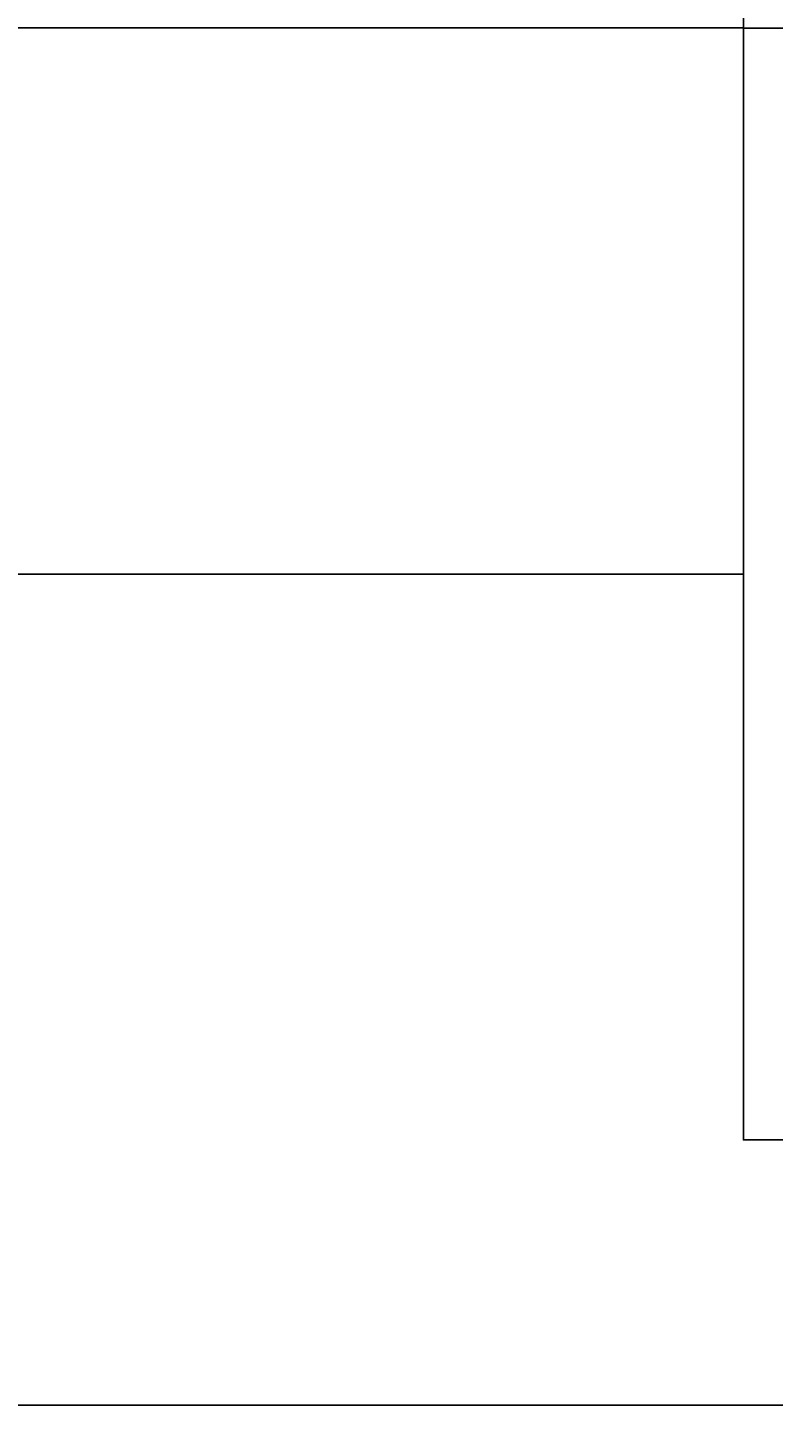
# Model space of a CAD drawing. Units: inches. Extents: x 35362 to 73946, y 43607 to 67532.
# Tile 134 of 134: x 67834 to 68341, y 59170 to 60122. Entities that reach past the tile are written whole.
import ezdxf

# ---------------------------------------------------------------- set-up
doc = ezdxf.new("R2010")
doc.units = ezdxf.units.IN
doc.header["$MEASUREMENT"] = 0
for name, color, linetype, lineweight in [('A-ANNO-DIMS', 2, 'Continuous', 18), ('E-SYMB', 1, 'Continuous', 25), ('E-WIRE', 3, 'Continuous', 25)]:
    doc.layers.add(name, color=color, linetype=linetype, lineweight=lineweight)
doc.styles.get("Standard").update_dxf_attribs({"font": 'arial.ttf'})
doc.dimstyles.get("Standard").update_dxf_attribs({"dimtxt": 0.18, "dimasz": 0.18, "dimexe": 0.18, "dimexo": 0.0625, "dimgap": 0.09, "dimtad": 0, "dimtih": 1, "dimtoh": 1, "dimdec": 4, "dimzin": 0, "dimdsep": 46, "dimtxsty": 'Standard', "dimcen": 0.09, "dimadec": 0, "dimazin": 0, "dimtfac": 1, "dimtdec": 4, "dimtofl": 0, "dimtmove": 0, "dimatfit": 3, "dimfxl": 1, "dimtolj": 1, "dimtzin": 0, "dimarcsym": 0})

# ---------------------------------------------------------------- blocks, each defined once
blk = doc.blocks.new('*D8')
at = {"layer": 'A-ANNO-DIMS', "color": 0, "lineweight": -2, "transparency": 16777216}
for p, q in [((66271.28651900003, 65771.51172800003), (73945.82566600003, 65771.51172800003)), ((73945.64566600005, 65771.33172800003), (73945.64566600005, 59737.03093663782)), ((73945.64566600005, 53702.36633900002), (73945.64566600005, 59736.66713036224)), ((72185.70816600003, 53702.18633900003), (73945.82566600003, 53702.18633900003))]:
    blk.add_line(p, q, dxfattribs=at)
at = {"layer": 'A-ANNO-DIMS', "color": 0, "transparency": 16777216}
for points in [[(73945.61566600006, 65771.33172800003), (73945.67566600005, 65771.33172800003), (73945.64566600005, 65771.51172800003)], [(73945.61566600006, 53702.36633900002), (73945.67566600005, 53702.36633900002), (73945.64566600005, 53702.18633900003)]]:
    blk.add_solid(points, dxfattribs=at)
at = {"layer": 'Defpoints', "color": 0, "transparency": 16777216}
for p in [(66271.22401900003, 65771.51172800003), (73945.64566600005, 65771.51172800003), (72185.64566600003, 53702.18633900003)]:
    blk.add_point(p, dxfattribs=at)
at = {"layer": 'A-ANNO-DIMS', "color": 0, "transparency": 16777216, "insert": (73945.64566600005, 59736.84903349999), "char_height": 0.18, "attachment_point": 5}
blk.add_mtext('\\A1;12069', dxfattribs=at)
blk = doc.blocks.new('*D10')
at = {"layer": 'A-ANNO-DIMS', "color": 0, "lineweight": -2, "transparency": 16777216}
for p, q in [((61240.96983600002, 59185.14395700003), (73945.82566600003, 59185.14395700003)), ((73945.64566600005, 59184.96395700003), (73945.64566600005, 56268.51827402935)), ((73945.64566600005, 53351.70866200003), (73945.64566600005, 56268.1543449707)), ((61240.96983600002, 53351.52866200003), (73945.82566600003, 53351.52866200003))]:
    blk.add_line(p, q, dxfattribs=at)
at = {"layer": 'A-ANNO-DIMS', "color": 0, "transparency": 16777216}
for points in [[(73945.61566600006, 59184.96395700003), (73945.67566600005, 59184.96395700003), (73945.64566600005, 59185.14395700003)], [(73945.61566600006, 53351.70866200003), (73945.67566600005, 53351.70866200003), (73945.64566600005, 53351.52866200003)]]:
    blk.add_solid(points, dxfattribs=at)
at = {"layer": 'Defpoints', "color": 0, "transparency": 16777216}
for p in [(61240.90733600002, 59185.14395700003), (61240.90733600002, 53351.52866200003), (73945.64566600005, 53351.52866200003)]:
    blk.add_point(p, dxfattribs=at)
at = {"layer": 'A-ANNO-DIMS', "color": 0, "transparency": 16777216, "insert": (73945.64566600005, 56268.33630949999), "char_height": 0.18, "attachment_point": 5}
blk.add_mtext('\\A1;5834', dxfattribs=at)
blk = doc.blocks.new('*D35')
at = {"layer": 'A-ANNO-DIMS', "color": 0, "lineweight": -2, "transparency": 16777216}
for p, q in [((61240.907336, 59185.206457), (61240.907336, 67531.691728)), ((61241.08733599999, 67531.51172799998), (64780.42646373397, 67531.51172799998)), ((68320.69076200001, 67531.51172799998), (64781.35163426603, 67531.51172799998)), ((68320.870762, 60122.408832), (68320.870762, 67531.691728))]:
    blk.add_line(p, q, dxfattribs=at)
at = {"layer": 'A-ANNO-DIMS', "color": 0, "transparency": 16777216}
for points in [[(61241.08733599999, 67531.541728), (61241.08733599999, 67531.481728), (61240.907336, 67531.51172799998)], [(68320.69076200001, 67531.541728), (68320.69076200001, 67531.481728), (68320.870762, 67531.51172799998)]]:
    blk.add_solid(points, dxfattribs=at)
at = {"layer": 'Defpoints', "color": 0, "transparency": 16777216}
for p in [(68320.870762, 67531.51172799998), (68320.870762, 60122.346332), (61240.907336, 59185.14395699999)]:
    blk.add_point(p, dxfattribs=at)
at = {"layer": 'A-ANNO-DIMS', "color": 0, "transparency": 16777216, "insert": (64780.889049, 67531.51172799998), "char_height": 0.18, "attachment_point": 5}
blk.add_mtext('\\A1;7080.0', dxfattribs=at)
blk = doc.blocks.new('*D36')
at = {"layer": 'A-ANNO-DIMS', "color": 0, "lineweight": -2, "transparency": 16777216}
for p, q in [((68320.80826200004, 60122.34633200002), (35361.76908500003, 60122.34633200002)), ((35361.94908500003, 60122.16633200002), (35361.94908500003, 57247.82893113781)), ((35361.94908500003, 54373.12772400002), (35361.94908500003, 57247.46512486223)), ((68320.80826200004, 54372.94772400003), (35361.76908500003, 54372.94772400002))]:
    blk.add_line(p, q, dxfattribs=at)
at = {"layer": 'A-ANNO-DIMS', "color": 0, "transparency": 16777216}
for points in [[(35361.91908500003, 60122.16633200002), (35361.97908500003, 60122.16633200002), (35361.94908500003, 60122.34633200002)], [(35361.91908500003, 54373.12772400002), (35361.97908500003, 54373.12772400002), (35361.94908500003, 54372.94772400002)]]:
    blk.add_solid(points, dxfattribs=at)
at = {"layer": 'Defpoints', "color": 0, "transparency": 16777216}
for p in [(68320.87076200004, 60122.34633200002), (35361.94908500003, 54372.94772400002), (68320.87076200004, 54372.94772400003)]:
    blk.add_point(p, dxfattribs=at)
at = {"layer": 'A-ANNO-DIMS', "color": 0, "transparency": 16777216, "insert": (35361.94908500004, 57247.64702799999), "char_height": 0.18, "attachment_point": 5}
blk.add_mtext('\\A1;5749.4', dxfattribs=at)
blk = doc.blocks.new('*D69')
at = {"layer": 'A-ANNO-DIMS', "color": 0, "lineweight": -2, "transparency": 16777216}
for p, q in [((68320.870762, 60122.408832), (68320.870762, 67531.691728)), ((68321.050762, 67531.51172799998), (69913.30289879469, 67531.51172799998)), ((71506.482539, 67531.51172799998), (69914.23040220531, 67531.51172799998)), ((71506.662539, 59451.647447), (71506.662539, 67531.691728))]:
    blk.add_line(p, q, dxfattribs=at)
at = {"layer": 'A-ANNO-DIMS', "color": 0, "transparency": 16777216}
for points in [[(68321.050762, 67531.541728), (68321.050762, 67531.481728), (68320.870762, 67531.51172799998)], [(71506.482539, 67531.541728), (71506.482539, 67531.481728), (71506.662539, 67531.51172799998)]]:
    blk.add_solid(points, dxfattribs=at)
at = {"layer": 'Defpoints', "color": 0, "transparency": 16777216}
for p in [(71506.662539, 67531.51172799998), (68320.870762, 60122.346332), (71506.662539, 59451.584947)]:
    blk.add_point(p, dxfattribs=at)
at = {"layer": 'A-ANNO-DIMS', "color": 0, "transparency": 16777216, "insert": (69913.76665050001, 67531.51172799998), "char_height": 0.18, "attachment_point": 5}
blk.add_mtext('\\A1;3185.8', dxfattribs=at)
blk = doc.blocks.new('*D70')
at = {"layer": 'A-ANNO-DIMS', "color": 0, "lineweight": -2, "transparency": 16777216}
for p, q in [((60785.27513900002, 64923.75242000003), (73945.82566600003, 64923.75242000003)), ((73945.64566600005, 64923.57242000003), (73945.64566600005, 62054.63015302935)), ((73945.64566600005, 59185.32395700003), (73945.64566600005, 62054.26622397069)), ((61240.96983600002, 59185.14395700003), (73945.82566600003, 59185.14395700003))]:
    blk.add_line(p, q, dxfattribs=at)
at = {"layer": 'A-ANNO-DIMS', "color": 0, "transparency": 16777216}
for points in [[(73945.61566600006, 64923.57242000003), (73945.67566600005, 64923.57242000003), (73945.64566600005, 64923.75242000003)], [(73945.61566600006, 59185.32395700003), (73945.67566600005, 59185.32395700003), (73945.64566600005, 59185.14395700003)]]:
    blk.add_solid(points, dxfattribs=at)
at = {"layer": 'Defpoints', "color": 0, "transparency": 16777216}
for p in [(60785.21263900002, 64923.75242000003), (73945.64566600005, 64923.75242000003), (61240.90733600002, 59185.14395700003)]:
    blk.add_point(p, dxfattribs=at)
at = {"layer": 'A-ANNO-DIMS', "color": 0, "transparency": 16777216, "insert": (73945.64566600005, 62054.44818849999), "char_height": 0.18, "attachment_point": 5}
blk.add_mtext('\\A1;5738.6', dxfattribs=at)
blk = doc.blocks.new('*D71')
at = {"layer": 'A-ANNO-DIMS', "color": 0, "lineweight": -2, "transparency": 16777216}
for p, q in [((63159.24181700003, 64828.55626700002), (73945.82566600003, 64828.55626700002)), ((73945.64566600005, 64828.37626700002), (73945.64566600005, 62007.03207652936)), ((73945.64566600005, 59185.32395700003), (73945.64566600005, 62006.6681474707)), ((61240.96983600002, 59185.14395700003), (73945.82566600003, 59185.14395700003))]:
    blk.add_line(p, q, dxfattribs=at)
at = {"layer": 'A-ANNO-DIMS', "color": 0, "transparency": 16777216}
for points in [[(73945.61566600006, 64828.37626700002), (73945.67566600005, 64828.37626700002), (73945.64566600005, 64828.55626700002)], [(73945.61566600006, 59185.32395700003), (73945.67566600005, 59185.32395700003), (73945.64566600005, 59185.14395700003)]]:
    blk.add_solid(points, dxfattribs=at)
at = {"layer": 'Defpoints', "color": 0, "transparency": 16777216}
for p in [(63159.17931700003, 64828.55626700002), (73945.64566600005, 64828.55626700002), (61240.90733600002, 59185.14395700003)]:
    blk.add_point(p, dxfattribs=at)
at = {"layer": 'A-ANNO-DIMS', "color": 0, "transparency": 16777216, "insert": (73945.64566600005, 62006.85011199999), "char_height": 0.18, "attachment_point": 5}
blk.add_mtext('\\A1;5643.4', dxfattribs=at)

msp = doc.modelspace()

# ---------------------------------------------------------------- linework, layer by layer
at = {"layer": 'E-SYMB'}
msp.add_lwpolyline([(68320.87076221016, 60122.34633153839), (68737.80188109005, 60122.34633153839), (68737.80188109005, 59365.72803786365), (68320.87076221016, 59365.72803786365)], close=True, dxfattribs=at)
at = {"layer": 'E-WIRE'}
msp.add_line((68320.87076221016, 59750.68874003685), (64849.6346681835, 59750.68874003685), dxfattribs=at)

# ---------------------------------------------------------------- dimensions: what is measured, and where the dimension line sits
at = {"layer": 'A-ANNO-DIMS'}
for base, p1, p2, picture, middle in [((68320.870762, 67531.51172799998), (61240.907336, 59185.14395699999), (68320.870762, 60122.346332), '*D35', (64780.889049, 67531.51172799998)), ((71506.662539, 67531.51172799998), (68320.870762, 60122.346332), (71506.662539, 59451.584947), '*D69', (69913.76665050001, 67531.51172799998))]:
    dim = msp.add_linear_dim(base=base, p1=p1, p2=p2, dimstyle='Standard', override={"dimdec": 1, "dimlfac": 1, "dimrnd": 0, "dimzin": 0, "dimdsep": 46, "dimlunit": 2}, dxfattribs=at)
    dim.commit()
    dim.dimension.update_dxf_attribs({"geometry": picture, "text_midpoint": middle})
for base, p1, p2, override, picture, middle in [((73945.64566600005, 65771.51172800003), (72185.645666, 53702.186339), (66271.224019, 65771.51172799998), {"dimdec": 0, "dimlfac": 1, "dimrnd": 0, "dimzin": 0, "dimdsep": 46, "dimlunit": 2}, '*D8', (73945.64566600005, 59736.84903349999)), ((73945.64566600005, 64923.75242000003), (61240.907336, 59185.14395699999), (60785.21263899999, 64923.75241999999), {"dimdec": 1, "dimlfac": 1, "dimrnd": 0, "dimzin": 0, "dimdsep": 46, "dimlunit": 2}, '*D70', (73945.64566600005, 62054.44818849999)), ((73945.64566600005, 64828.55626700002), (61240.907336, 59185.14395699999), (63159.179317, 64828.556267), {"dimdec": 1, "dimlfac": 1, "dimrnd": 0, "dimzin": 0, "dimdsep": 46, "dimlunit": 2}, '*D71', (73945.64566600005, 62006.85011199999)), ((35361.94908500003, 54372.94772400002), (68320.870762, 60122.346332), (68320.870762, 54372.947724), {"dimdec": 1, "dimlfac": 1, "dimrnd": 0, "dimzin": 0, "dimdsep": 46, "dimlunit": 2}, '*D36', (35361.94908500004, 57247.64702799999)), ((73945.64566600005, 53351.52866200003), (61240.907336, 59185.14395699999), (61240.907336, 53351.52866199999), {"dimdec": 0, "dimlfac": 1, "dimrnd": 0, "dimzin": 0, "dimdsep": 46, "dimlunit": 2}, '*D10', (73945.64566600005, 56268.33630949999))]:
    dim = msp.add_linear_dim(base=base, p1=p1, p2=p2, angle=90, dimstyle='Standard', override=override, dxfattribs=at)
    dim.commit()
    dim.dimension.update_dxf_attribs({"geometry": picture, "text_midpoint": middle})

doc.saveas('drawing.dxf')
